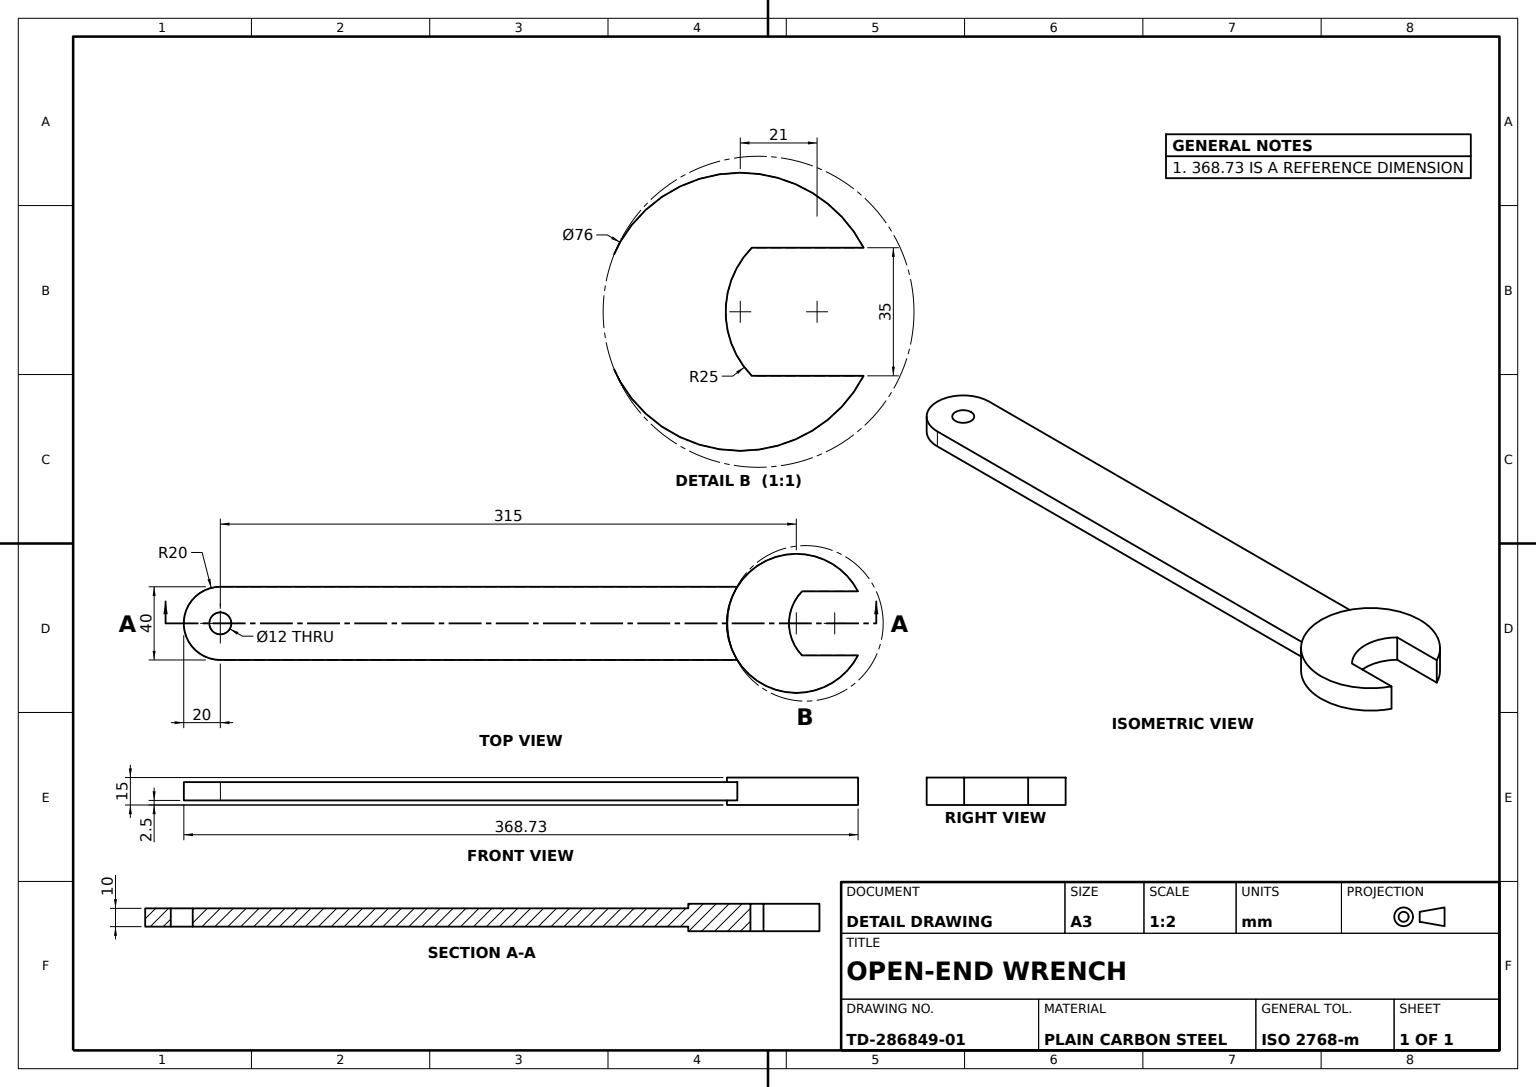
SolidWorks part; units mm, degrees
material "Plain Carbon Steel"
ref_plane "Front Plane" through (0, 0, 0) normal (0, 0, 1) x (1, 0, 0)
ref_plane "Top Plane" through (0, 0, 0) normal (0, 1, 0) x (1, 0, 0)
ref_plane "Right Plane" through (0, 0, 0) normal (1, 0, 0) x (0, 0, -1)
sketch "Wrench Outline Sketch" plane through (0, 0, 0) normal (0, 1, 0) x (1, 0, 0)
  line L0 (-157.5, 0) -> (157.5, 0) construction
  line L1 (-157.5, 20) -> (125.189, 20)
  line L2 (-157.5, -20) -> (125.189, -20)
  line L4 (160.6464, 17.5) -> (191.2305, 17.5)
  line L6 (160.6464, -17.5) -> (191.2305, -17.5)
  line L8 (155.2012, 9.0646) -> (194.9567, -6.4026) construction
  line L9 (155.2012, -9.0646) -> (194.9567, 6.4026) construction
  arc A0 (-157.5, 20) -> (-157.5, -20) centre (-157.5, 0) ccw
  arc A2 (191.2305, 17.5) -> (191.2305, -17.5) centre (157.5, 0) ccw
  arc A3 (160.6464, 17.5) -> (160.6464, -17.5) centre (178.5, 0) ccw
  arc A4 (177.4962, -0.3905) -> (177.4962, 0.3905) centre (157.5, 0) ccw
  circle A5 centre (-157.5, 0) radius 6
  point P2 (0, 0)
  dimension "D2" = 20
  dimension "D3" = 76
  dimension "D4" = 50
  dimension "D5" = 21
  dimension "D6" = 12
  dimension "D1" = 315
  dimension "D7" = 312.7012
  dimension "D8" = 318.1464
extrude "Wrench Handle 10mm" add sketch "Wrench Outline Sketch" along normal mid plane 10 contours A2 L1 A0 L2 A5
sketch "Jaw Head Sketch" plane through (0, 0, 0) normal (0, 1, 0) x (1, 0, 0)
  line L0 (160.6464, -17.5) -> (191.2305, -17.5) construction
  line L1 (160.6464, 17.5) -> (191.2305, 17.5) construction
  line L2 (160.6464, -17.5) -> (191.2305, -17.5)
  line L3 (160.6464, 17.5) -> (191.2305, 17.5)
  arc A0 (160.6464, 17.5) -> (160.6464, -17.5) centre (178.5, 0) ccw construction
  arc A1 (191.2305, 17.5) -> (191.2305, -17.5) centre (157.5, 0) ccw construction
  arc A2 (160.6464, 17.5) -> (160.6464, -17.5) centre (178.5, 0) ccw
  arc A3 (191.2305, 17.5) -> (191.2305, -17.5) centre (157.5, 0) ccw
extrude "Jaw Head Boss 15mm" add sketch "Jaw Head Sketch" along normal mid plane 15
